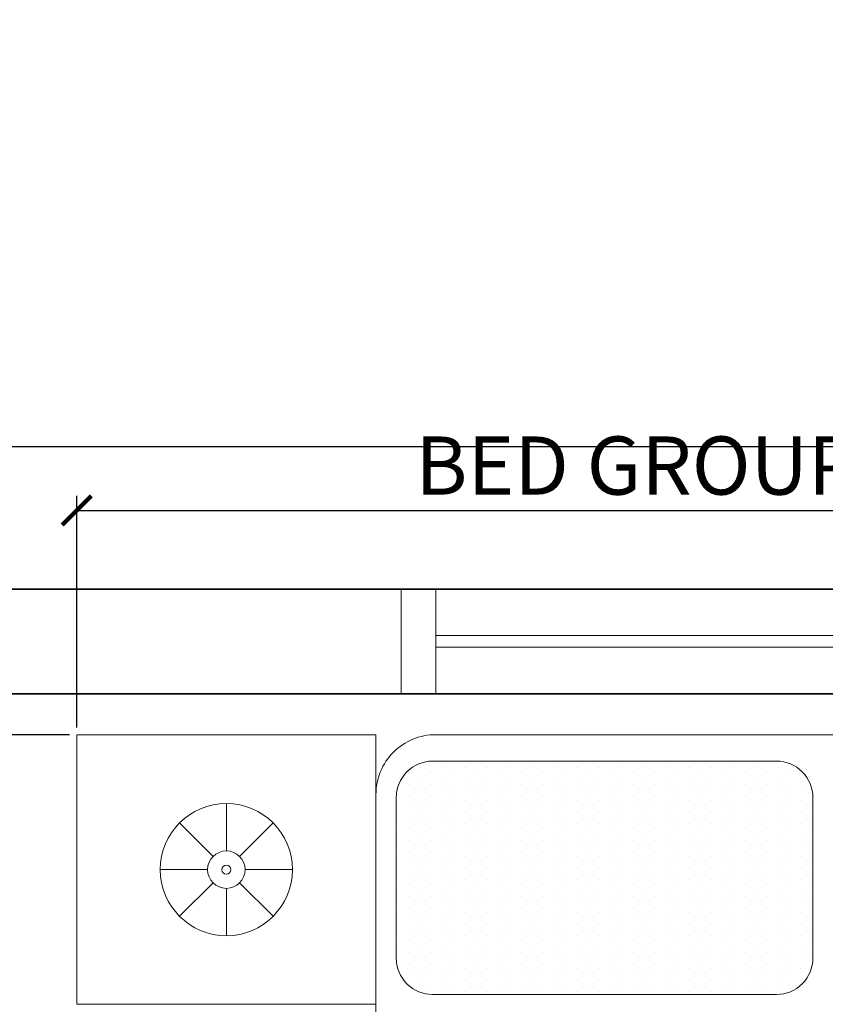
# Model space of a CAD drawing. Units: inches. Extents: x 3283068 to 3284536, y 3240756 to 3241803.
# Tile 10 of 19: x 3283383 to 3283453, y 3241603 to 3241688. Entities that reach past the tile are written whole.
import ezdxf

# ---------------------------------------------------------------- set-up
doc = ezdxf.new("R2010")
doc.units = ezdxf.units.IN
for name, color, linetype, lineweight in [('A-ANNO-DIMS', 2, 'Continuous', 18), ('furniture', 40, 'Continuous', 18), ('wall', 20, 'Continuous', 35), ('window', 100, 'Continuous', 18)]:
    doc.layers.add(name, color=color, linetype=linetype, lineweight=lineweight)
doc.styles.get("Standard").update_dxf_attribs({"font": 'arial.ttf'})
doc.dimstyles.new('ISO-25', dxfattribs={"dimtxt": 5, "dimasz": 2.5, "dimexe": 1.25, "dimexo": 0.625, "dimtad": 1, "dimlunit": 4, "dimtxsty": 'Standard', "dimblk": 'ARCHTICK', "dimcen": 2.5, "dimadec": 0, "dimazin": 0, "dimtfac": 1, "dimtmove": 0, "dimatfit": 3, "dimfxl": 1, "dimarcsym": 0})

# ---------------------------------------------------------------- blocks, each defined once
blk = doc.blocks.new('*X12')
at = {"color": 0}
for p, q in [((266.25, 456.9375), (266.25, 456.9375)), ((266.4375, 457.03125), (266.4375, 457.03125)), ((266.625, 456.9375), (266.625, 456.9375)), ((266.8125, 457.03125), (266.8125, 457.03125)), ((267, 456.9375), (267, 456.9375)), ((267.1875, 457.03125), (267.1875, 457.03125)), ((267.375, 456.9375), (267.375, 456.9375)), ((267.5625, 457.03125), (267.5625, 457.03125)), ((267.75, 456.9375), (267.75, 456.9375)), ((267.9375, 457.03125), (267.9375, 457.03125)), ((268.125, 456.9375), (268.125, 456.9375)), ((268.3125, 457.03125), (268.3125, 457.03125)), ((268.5, 456.9375), (268.5, 456.9375)), ((268.6875, 457.03125), (268.6875, 457.03125)), ((268.875, 456.9375), (268.875, 456.9375)), ((269.0625, 457.03125), (269.0625, 457.03125)), ((269.25, 456.9375), (269.25, 456.9375)), ((269.4375, 457.03125), (269.4375, 457.03125)), ((269.625, 456.9375), (269.625, 456.9375)), ((269.8125, 457.03125), (269.8125, 457.03125)), ((270, 456.9375), (270, 456.9375)), ((270.1875, 457.03125), (270.1875, 457.03125)), ((270.375, 456.9375), (270.375, 456.9375)), ((270.5625, 457.03125), (270.5625, 457.03125)), ((270.75, 456.9375), (270.75, 456.9375)), ((270.9375, 457.03125), (270.9375, 457.03125)), ((271.125, 456.9375), (271.125, 456.9375)), ((271.3125, 457.03125), (271.3125, 457.03125)), ((271.5, 456.9375), (271.5, 456.9375)), ((271.6875, 457.03125), (271.6875, 457.03125)), ((271.875, 456.9375), (271.875, 456.9375)), ((272.0625, 457.03125), (272.0625, 457.03125)), ((272.25, 456.9375), (272.25, 456.9375)), ((266.0625, 456.84375), (266.0625, 456.84375)), ((266.25, 456.75), (266.25, 456.75)), ((266.4375, 456.84375), (266.4375, 456.84375)), ((266.625, 456.75), (266.625, 456.75)), ((266.8125, 456.84375), (266.8125, 456.84375)), ((267, 456.75), (267, 456.75)), ((267.1875, 456.84375), (267.1875, 456.84375)), ((267.375, 456.75), (267.375, 456.75)), ((267.5625, 456.84375), (267.5625, 456.84375)), ((267.75, 456.75), (267.75, 456.75)), ((267.9375, 456.84375), (267.9375, 456.84375)), ((268.125, 456.75), (268.125, 456.75)), ((268.3125, 456.84375), (268.3125, 456.84375)), ((268.5, 456.75), (268.5, 456.75)), ((268.6875, 456.84375), (268.6875, 456.84375)), ((268.875, 456.75), (268.875, 456.75)), ((269.0625, 456.84375), (269.0625, 456.84375)), ((269.25, 456.75), (269.25, 456.75)), ((269.4375, 456.84375), (269.4375, 456.84375)), ((269.625, 456.75), (269.625, 456.75)), ((269.8125, 456.84375), (269.8125, 456.84375)), ((270, 456.75), (270, 456.75)), ((270.1875, 456.84375), (270.1875, 456.84375)), ((270.375, 456.75), (270.375, 456.75)), ((270.5625, 456.84375), (270.5625, 456.84375)), ((270.75, 456.75), (270.75, 456.75)), ((270.9375, 456.84375), (270.9375, 456.84375)), ((271.125, 456.75), (271.125, 456.75)), ((271.3125, 456.84375), (271.3125, 456.84375)), ((271.5, 456.75), (271.5, 456.75)), ((271.6875, 456.84375), (271.6875, 456.84375)), ((271.875, 456.75), (271.875, 456.75)), ((272.0625, 456.84375), (272.0625, 456.84375)), ((272.25, 456.75), (272.25, 456.75)), ((272.4375, 456.84375), (272.4375, 456.84375)), ((272.625, 456.75), (272.625, 456.75)), ((266.0625, 456.65625), (266.0625, 456.65625)), ((266.4375, 456.65625), (266.4375, 456.65625)), ((266.8125, 456.65625), (266.8125, 456.65625)), ((267.1875, 456.65625), (267.1875, 456.65625)), ((267.5625, 456.65625), (267.5625, 456.65625)), ((267.9375, 456.65625), (267.9375, 456.65625)), ((268.3125, 456.65625), (268.3125, 456.65625)), ((268.6875, 456.65625), (268.6875, 456.65625)), ((269.0625, 456.65625), (269.0625, 456.65625)), ((269.4375, 456.65625), (269.4375, 456.65625)), ((269.8125, 456.65625), (269.8125, 456.65625)), ((270.1875, 456.65625), (270.1875, 456.65625)), ((270.5625, 456.65625), (270.5625, 456.65625)), ((270.9375, 456.65625), (270.9375, 456.65625)), ((271.3125, 456.65625), (271.3125, 456.65625)), ((271.6875, 456.65625), (271.6875, 456.65625)), ((272.0625, 456.65625), (272.0625, 456.65625)), ((272.4375, 456.65625), (272.4375, 456.65625)), ((265.875, 456.5625), (265.875, 456.5625)), ((266.0625, 456.46875), (266.0625, 456.46875)), ((266.25, 456.5625), (266.25, 456.5625)), ((266.4375, 456.46875), (266.4375, 456.46875)), ((266.625, 456.5625), (266.625, 456.5625)), ((266.8125, 456.46875), (266.8125, 456.46875)), ((267, 456.5625), (267, 456.5625)), ((267.1875, 456.46875), (267.1875, 456.46875)), ((267.375, 456.5625), (267.375, 456.5625)), ((267.5625, 456.46875), (267.5625, 456.46875)), ((267.75, 456.5625), (267.75, 456.5625)), ((267.9375, 456.46875), (267.9375, 456.46875)), ((268.125, 456.5625), (268.125, 456.5625)), ((268.3125, 456.46875), (268.3125, 456.46875)), ((268.5, 456.5625), (268.5, 456.5625)), ((268.6875, 456.46875), (268.6875, 456.46875)), ((268.875, 456.5625), (268.875, 456.5625)), ((269.0625, 456.46875), (269.0625, 456.46875)), ((269.25, 456.5625), (269.25, 456.5625)), ((269.4375, 456.46875), (269.4375, 456.46875)), ((269.625, 456.5625), (269.625, 456.5625)), ((269.8125, 456.46875), (269.8125, 456.46875)), ((270, 456.5625), (270, 456.5625)), ((270.1875, 456.46875), (270.1875, 456.46875)), ((270.375, 456.5625), (270.375, 456.5625)), ((270.5625, 456.46875), (270.5625, 456.46875)), ((270.75, 456.5625), (270.75, 456.5625)), ((270.9375, 456.46875), (270.9375, 456.46875)), ((271.125, 456.5625), (271.125, 456.5625)), ((271.3125, 456.46875), (271.3125, 456.46875)), ((271.5, 456.5625), (271.5, 456.5625)), ((271.6875, 456.46875), (271.6875, 456.46875)), ((271.875, 456.5625), (271.875, 456.5625)), ((272.0625, 456.46875), (272.0625, 456.46875)), ((272.25, 456.5625), (272.25, 456.5625)), ((272.4375, 456.46875), (272.4375, 456.46875)), ((272.625, 456.5625), (272.625, 456.5625)), ((272.8125, 456.46875), (272.8125, 456.46875)), ((265.875, 456.375), (265.875, 456.375)), ((266.0625, 456.28125), (266.0625, 456.28125)), ((266.25, 456.375), (266.25, 456.375)), ((266.4375, 456.28125), (266.4375, 456.28125)), ((266.625, 456.375), (266.625, 456.375)), ((266.8125, 456.28125), (266.8125, 456.28125)), ((267, 456.375), (267, 456.375)), ((267.1875, 456.28125), (267.1875, 456.28125)), ((267.375, 456.375), (267.375, 456.375)), ((267.5625, 456.28125), (267.5625, 456.28125)), ((267.75, 456.375), (267.75, 456.375)), ((267.9375, 456.28125), (267.9375, 456.28125)), ((268.125, 456.375), (268.125, 456.375)), ((268.3125, 456.28125), (268.3125, 456.28125)), ((268.5, 456.375), (268.5, 456.375)), ((268.6875, 456.28125), (268.6875, 456.28125)), ((268.875, 456.375), (268.875, 456.375)), ((269.0625, 456.28125), (269.0625, 456.28125)), ((269.25, 456.375), (269.25, 456.375)), ((269.4375, 456.28125), (269.4375, 456.28125)), ((269.625, 456.375), (269.625, 456.375)), ((269.8125, 456.28125), (269.8125, 456.28125)), ((270, 456.375), (270, 456.375)), ((270.1875, 456.28125), (270.1875, 456.28125)), ((270.375, 456.375), (270.375, 456.375)), ((270.5625, 456.28125), (270.5625, 456.28125)), ((270.75, 456.375), (270.75, 456.375)), ((270.9375, 456.28125), (270.9375, 456.28125)), ((271.125, 456.375), (271.125, 456.375)), ((271.3125, 456.28125), (271.3125, 456.28125)), ((271.5, 456.375), (271.5, 456.375)), ((271.6875, 456.28125), (271.6875, 456.28125)), ((271.875, 456.375), (271.875, 456.375)), ((272.0625, 456.28125), (272.0625, 456.28125)), ((272.25, 456.375), (272.25, 456.375)), ((272.4375, 456.28125), (272.4375, 456.28125)), ((272.625, 456.375), (272.625, 456.375)), ((272.8125, 456.28125), (272.8125, 456.28125)), ((265.875, 456.1875), (265.875, 456.1875)), ((266.0625, 456.09375), (266.0625, 456.09375)), ((266.25, 456.1875), (266.25, 456.1875)), ((266.4375, 456.09375), (266.4375, 456.09375)), ((266.625, 456.1875), (266.625, 456.1875)), ((266.8125, 456.09375), (266.8125, 456.09375)), ((267, 456.1875), (267, 456.1875)), ((267.1875, 456.09375), (267.1875, 456.09375)), ((267.375, 456.1875), (267.375, 456.1875)), ((267.5625, 456.09375), (267.5625, 456.09375)), ((267.75, 456.1875), (267.75, 456.1875)), ((267.9375, 456.09375), (267.9375, 456.09375)), ((268.125, 456.1875), (268.125, 456.1875)), ((268.3125, 456.09375), (268.3125, 456.09375)), ((268.5, 456.1875), (268.5, 456.1875)), ((268.6875, 456.09375), (268.6875, 456.09375)), ((268.875, 456.1875), (268.875, 456.1875)), ((269.0625, 456.09375), (269.0625, 456.09375)), ((269.25, 456.1875), (269.25, 456.1875)), ((269.4375, 456.09375), (269.4375, 456.09375)), ((269.625, 456.1875), (269.625, 456.1875)), ((269.8125, 456.09375), (269.8125, 456.09375)), ((270, 456.1875), (270, 456.1875)), ((270.1875, 456.09375), (270.1875, 456.09375)), ((270.375, 456.1875), (270.375, 456.1875)), ((270.5625, 456.09375), (270.5625, 456.09375)), ((270.75, 456.1875), (270.75, 456.1875)), ((270.9375, 456.09375), (270.9375, 456.09375)), ((271.125, 456.1875), (271.125, 456.1875)), ((271.3125, 456.09375), (271.3125, 456.09375)), ((271.5, 456.1875), (271.5, 456.1875)), ((271.6875, 456.09375), (271.6875, 456.09375)), ((271.875, 456.1875), (271.875, 456.1875)), ((272.0625, 456.09375), (272.0625, 456.09375)), ((272.25, 456.1875), (272.25, 456.1875)), ((272.4375, 456.09375), (272.4375, 456.09375)), ((272.625, 456.1875), (272.625, 456.1875)), ((272.8125, 456.09375), (272.8125, 456.09375)), ((265.875, 456), (265.875, 456)), ((266.25, 456), (266.25, 456)), ((266.625, 456), (266.625, 456)), ((267, 456), (267, 456)), ((267.375, 456), (267.375, 456)), ((267.75, 456), (267.75, 456)), ((268.125, 456), (268.125, 456)), ((268.5, 456), (268.5, 456)), ((268.875, 456), (268.875, 456)), ((269.25, 456), (269.25, 456)), ((269.625, 456), (269.625, 456)), ((270, 456), (270, 456)), ((270.375, 456), (270.375, 456)), ((270.75, 456), (270.75, 456)), ((271.125, 456), (271.125, 456)), ((271.5, 456), (271.5, 456)), ((271.875, 456), (271.875, 456)), ((272.25, 456), (272.25, 456)), ((272.625, 456), (272.625, 456)), ((265.875, 455.8125), (265.875, 455.8125)), ((266.0625, 455.90625), (266.0625, 455.90625)), ((266.25, 455.8125), (266.25, 455.8125)), ((266.4375, 455.90625), (266.4375, 455.90625)), ((266.625, 455.8125), (266.625, 455.8125)), ((266.8125, 455.90625), (266.8125, 455.90625)), ((267, 455.8125), (267, 455.8125)), ((267.1875, 455.90625), (267.1875, 455.90625)), ((267.375, 455.8125), (267.375, 455.8125)), ((267.5625, 455.90625), (267.5625, 455.90625)), ((267.75, 455.8125), (267.75, 455.8125)), ((267.9375, 455.90625), (267.9375, 455.90625)), ((268.125, 455.8125), (268.125, 455.8125)), ((268.3125, 455.90625), (268.3125, 455.90625)), ((268.5, 455.8125), (268.5, 455.8125)), ((268.6875, 455.90625), (268.6875, 455.90625)), ((268.875, 455.8125), (268.875, 455.8125)), ((269.0625, 455.90625), (269.0625, 455.90625)), ((269.25, 455.8125), (269.25, 455.8125)), ((269.4375, 455.90625), (269.4375, 455.90625)), ((269.625, 455.8125), (269.625, 455.8125)), ((269.8125, 455.90625), (269.8125, 455.90625)), ((270, 455.8125), (270, 455.8125)), ((270.1875, 455.90625), (270.1875, 455.90625)), ((270.375, 455.8125), (270.375, 455.8125)), ((270.5625, 455.90625), (270.5625, 455.90625)), ((270.75, 455.8125), (270.75, 455.8125)), ((270.9375, 455.90625), (270.9375, 455.90625)), ((271.125, 455.8125), (271.125, 455.8125)), ((271.3125, 455.90625), (271.3125, 455.90625)), ((271.5, 455.8125), (271.5, 455.8125)), ((271.6875, 455.90625), (271.6875, 455.90625)), ((271.875, 455.8125), (271.875, 455.8125)), ((272.0625, 455.90625), (272.0625, 455.90625)), ((272.25, 455.8125), (272.25, 455.8125)), ((272.4375, 455.90625), (272.4375, 455.90625)), ((272.625, 455.8125), (272.625, 455.8125)), ((272.8125, 455.90625), (272.8125, 455.90625)), ((265.875, 455.625), (265.875, 455.625)), ((266.0625, 455.71875), (266.0625, 455.71875)), ((266.25, 455.625), (266.25, 455.625)), ((266.4375, 455.71875), (266.4375, 455.71875)), ((266.625, 455.625), (266.625, 455.625)), ((266.8125, 455.71875), (266.8125, 455.71875)), ((267, 455.625), (267, 455.625)), ((267.1875, 455.71875), (267.1875, 455.71875)), ((267.375, 455.625), (267.375, 455.625)), ((267.5625, 455.71875), (267.5625, 455.71875)), ((267.75, 455.625), (267.75, 455.625)), ((267.9375, 455.71875), (267.9375, 455.71875)), ((268.125, 455.625), (268.125, 455.625)), ((268.3125, 455.71875), (268.3125, 455.71875)), ((268.5, 455.625), (268.5, 455.625)), ((268.6875, 455.71875), (268.6875, 455.71875)), ((268.875, 455.625), (268.875, 455.625)), ((269.0625, 455.71875), (269.0625, 455.71875)), ((269.25, 455.625), (269.25, 455.625)), ((269.4375, 455.71875), (269.4375, 455.71875)), ((269.625, 455.625), (269.625, 455.625)), ((269.8125, 455.71875), (269.8125, 455.71875)), ((270, 455.625), (270, 455.625)), ((270.1875, 455.71875), (270.1875, 455.71875)), ((270.375, 455.625), (270.375, 455.625)), ((270.5625, 455.71875), (270.5625, 455.71875)), ((270.75, 455.625), (270.75, 455.625)), ((270.9375, 455.71875), (270.9375, 455.71875)), ((271.125, 455.625), (271.125, 455.625)), ((271.3125, 455.71875), (271.3125, 455.71875)), ((271.5, 455.625), (271.5, 455.625)), ((271.6875, 455.71875), (271.6875, 455.71875)), ((271.875, 455.625), (271.875, 455.625)), ((272.0625, 455.71875), (272.0625, 455.71875)), ((272.25, 455.625), (272.25, 455.625)), ((272.4375, 455.71875), (272.4375, 455.71875)), ((272.625, 455.625), (272.625, 455.625)), ((272.8125, 455.71875), (272.8125, 455.71875)), ((265.875, 455.4375), (265.875, 455.4375)), ((266.0625, 455.53125), (266.0625, 455.53125)), ((266.25, 455.4375), (266.25, 455.4375)), ((266.4375, 455.53125), (266.4375, 455.53125)), ((266.625, 455.4375), (266.625, 455.4375)), ((266.8125, 455.53125), (266.8125, 455.53125)), ((267, 455.4375), (267, 455.4375)), ((267.1875, 455.53125), (267.1875, 455.53125)), ((267.375, 455.4375), (267.375, 455.4375)), ((267.5625, 455.53125), (267.5625, 455.53125)), ((267.75, 455.4375), (267.75, 455.4375)), ((267.9375, 455.53125), (267.9375, 455.53125)), ((268.125, 455.4375), (268.125, 455.4375)), ((268.3125, 455.53125), (268.3125, 455.53125)), ((268.5, 455.4375), (268.5, 455.4375)), ((268.6875, 455.53125), (268.6875, 455.53125)), ((268.875, 455.4375), (268.875, 455.4375)), ((269.0625, 455.53125), (269.0625, 455.53125)), ((269.25, 455.4375), (269.25, 455.4375)), ((269.4375, 455.53125), (269.4375, 455.53125)), ((269.625, 455.4375), (269.625, 455.4375)), ((269.8125, 455.53125), (269.8125, 455.53125)), ((270, 455.4375), (270, 455.4375)), ((270.1875, 455.53125), (270.1875, 455.53125)), ((270.375, 455.4375), (270.375, 455.4375)), ((270.5625, 455.53125), (270.5625, 455.53125)), ((270.75, 455.4375), (270.75, 455.4375)), ((270.9375, 455.53125), (270.9375, 455.53125)), ((271.125, 455.4375), (271.125, 455.4375)), ((271.3125, 455.53125), (271.3125, 455.53125)), ((271.5, 455.4375), (271.5, 455.4375)), ((271.6875, 455.53125), (271.6875, 455.53125)), ((271.875, 455.4375), (271.875, 455.4375)), ((272.0625, 455.53125), (272.0625, 455.53125)), ((272.25, 455.4375), (272.25, 455.4375)), ((272.4375, 455.53125), (272.4375, 455.53125)), ((272.625, 455.4375), (272.625, 455.4375)), ((272.8125, 455.53125), (272.8125, 455.53125)), ((266.0625, 455.34375), (266.0625, 455.34375)), ((266.4375, 455.34375), (266.4375, 455.34375)), ((266.8125, 455.34375), (266.8125, 455.34375)), ((267.1875, 455.34375), (267.1875, 455.34375)), ((267.5625, 455.34375), (267.5625, 455.34375)), ((267.9375, 455.34375), (267.9375, 455.34375)), ((268.3125, 455.34375), (268.3125, 455.34375)), ((268.6875, 455.34375), (268.6875, 455.34375)), ((269.0625, 455.34375), (269.0625, 455.34375)), ((269.4375, 455.34375), (269.4375, 455.34375)), ((269.8125, 455.34375), (269.8125, 455.34375)), ((270.1875, 455.34375), (270.1875, 455.34375)), ((270.5625, 455.34375), (270.5625, 455.34375)), ((270.9375, 455.34375), (270.9375, 455.34375)), ((271.3125, 455.34375), (271.3125, 455.34375)), ((271.6875, 455.34375), (271.6875, 455.34375)), ((272.0625, 455.34375), (272.0625, 455.34375)), ((272.4375, 455.34375), (272.4375, 455.34375)), ((272.8125, 455.34375), (272.8125, 455.34375)), ((265.875, 455.25), (265.875, 455.25)), ((266.0625, 455.15625), (266.0625, 455.15625)), ((266.25, 455.25), (266.25, 455.25)), ((266.4375, 455.15625), (266.4375, 455.15625)), ((266.625, 455.25), (266.625, 455.25)), ((266.8125, 455.15625), (266.8125, 455.15625)), ((267, 455.25), (267, 455.25)), ((267.1875, 455.15625), (267.1875, 455.15625)), ((267.375, 455.25), (267.375, 455.25)), ((267.5625, 455.15625), (267.5625, 455.15625)), ((267.75, 455.25), (267.75, 455.25)), ((267.9375, 455.15625), (267.9375, 455.15625)), ((268.125, 455.25), (268.125, 455.25)), ((268.3125, 455.15625), (268.3125, 455.15625)), ((268.5, 455.25), (268.5, 455.25)), ((268.6875, 455.15625), (268.6875, 455.15625)), ((268.875, 455.25), (268.875, 455.25)), ((269.0625, 455.15625), (269.0625, 455.15625)), ((269.25, 455.25), (269.25, 455.25)), ((269.4375, 455.15625), (269.4375, 455.15625)), ((269.625, 455.25), (269.625, 455.25)), ((269.8125, 455.15625), (269.8125, 455.15625)), ((270, 455.25), (270, 455.25)), ((270.1875, 455.15625), (270.1875, 455.15625)), ((270.375, 455.25), (270.375, 455.25)), ((270.5625, 455.15625), (270.5625, 455.15625)), ((270.75, 455.25), (270.75, 455.25)), ((270.9375, 455.15625), (270.9375, 455.15625)), ((271.125, 455.25), (271.125, 455.25)), ((271.3125, 455.15625), (271.3125, 455.15625)), ((271.5, 455.25), (271.5, 455.25)), ((271.6875, 455.15625), (271.6875, 455.15625)), ((271.875, 455.25), (271.875, 455.25)), ((272.0625, 455.15625), (272.0625, 455.15625)), ((272.25, 455.25), (272.25, 455.25)), ((272.4375, 455.15625), (272.4375, 455.15625)), ((272.625, 455.25), (272.625, 455.25)), ((272.8125, 455.15625), (272.8125, 455.15625)), ((265.875, 455.0625), (265.875, 455.0625)), ((266.0625, 454.96875), (266.0625, 454.96875)), ((266.25, 455.0625), (266.25, 455.0625)), ((266.4375, 454.96875), (266.4375, 454.96875)), ((266.625, 455.0625), (266.625, 455.0625)), ((266.8125, 454.96875), (266.8125, 454.96875)), ((267, 455.0625), (267, 455.0625)), ((267.1875, 454.96875), (267.1875, 454.96875)), ((267.375, 455.0625), (267.375, 455.0625)), ((267.5625, 454.96875), (267.5625, 454.96875)), ((267.75, 455.0625), (267.75, 455.0625)), ((267.9375, 454.96875), (267.9375, 454.96875)), ((268.125, 455.0625), (268.125, 455.0625)), ((268.3125, 454.96875), (268.3125, 454.96875)), ((268.5, 455.0625), (268.5, 455.0625)), ((268.6875, 454.96875), (268.6875, 454.96875)), ((268.875, 455.0625), (268.875, 455.0625)), ((269.0625, 454.96875), (269.0625, 454.96875)), ((269.25, 455.0625), (269.25, 455.0625)), ((269.4375, 454.96875), (269.4375, 454.96875)), ((269.625, 455.0625), (269.625, 455.0625)), ((269.8125, 454.96875), (269.8125, 454.96875)), ((270, 455.0625), (270, 455.0625)), ((270.1875, 454.96875), (270.1875, 454.96875)), ((270.375, 455.0625), (270.375, 455.0625)), ((270.5625, 454.96875), (270.5625, 454.96875)), ((270.75, 455.0625), (270.75, 455.0625)), ((270.9375, 454.96875), (270.9375, 454.96875)), ((271.125, 455.0625), (271.125, 455.0625)), ((271.3125, 454.96875), (271.3125, 454.96875)), ((271.5, 455.0625), (271.5, 455.0625)), ((271.6875, 454.96875), (271.6875, 454.96875)), ((271.875, 455.0625), (271.875, 455.0625)), ((272.0625, 454.96875), (272.0625, 454.96875)), ((272.25, 455.0625), (272.25, 455.0625)), ((272.4375, 454.96875), (272.4375, 454.96875)), ((272.625, 455.0625), (272.625, 455.0625)), ((272.8125, 454.96875), (272.8125, 454.96875)), ((265.875, 454.875), (265.875, 454.875)), ((266.0625, 454.78125), (266.0625, 454.78125)), ((266.25, 454.875), (266.25, 454.875)), ((266.4375, 454.78125), (266.4375, 454.78125)), ((266.625, 454.875), (266.625, 454.875)), ((266.8125, 454.78125), (266.8125, 454.78125)), ((267, 454.875), (267, 454.875)), ((267.1875, 454.78125), (267.1875, 454.78125)), ((267.375, 454.875), (267.375, 454.875)), ((267.5625, 454.78125), (267.5625, 454.78125)), ((267.75, 454.875), (267.75, 454.875)), ((267.9375, 454.78125), (267.9375, 454.78125)), ((268.125, 454.875), (268.125, 454.875)), ((268.3125, 454.78125), (268.3125, 454.78125)), ((268.5, 454.875), (268.5, 454.875)), ((268.6875, 454.78125), (268.6875, 454.78125)), ((268.875, 454.875), (268.875, 454.875)), ((269.0625, 454.78125), (269.0625, 454.78125)), ((269.25, 454.875), (269.25, 454.875)), ((269.4375, 454.78125), (269.4375, 454.78125)), ((269.625, 454.875), (269.625, 454.875)), ((269.8125, 454.78125), (269.8125, 454.78125)), ((270, 454.875), (270, 454.875)), ((270.1875, 454.78125), (270.1875, 454.78125)), ((270.375, 454.875), (270.375, 454.875)), ((270.5625, 454.78125), (270.5625, 454.78125)), ((270.75, 454.875), (270.75, 454.875)), ((270.9375, 454.78125), (270.9375, 454.78125)), ((271.125, 454.875), (271.125, 454.875)), ((271.3125, 454.78125), (271.3125, 454.78125)), ((271.5, 454.875), (271.5, 454.875)), ((271.6875, 454.78125), (271.6875, 454.78125)), ((271.875, 454.875), (271.875, 454.875)), ((272.0625, 454.78125), (272.0625, 454.78125)), ((272.25, 454.875), (272.25, 454.875)), ((272.4375, 454.78125), (272.4375, 454.78125)), ((272.625, 454.875), (272.625, 454.875)), ((272.8125, 454.78125), (272.8125, 454.78125)), ((265.875, 454.6875), (265.875, 454.6875)), ((266.25, 454.6875), (266.25, 454.6875)), ((266.625, 454.6875), (266.625, 454.6875)), ((267, 454.6875), (267, 454.6875)), ((267.375, 454.6875), (267.375, 454.6875)), ((267.75, 454.6875), (267.75, 454.6875)), ((268.125, 454.6875), (268.125, 454.6875)), ((268.5, 454.6875), (268.5, 454.6875)), ((268.875, 454.6875), (268.875, 454.6875)), ((269.25, 454.6875), (269.25, 454.6875)), ((269.625, 454.6875), (269.625, 454.6875)), ((270, 454.6875), (270, 454.6875)), ((270.375, 454.6875), (270.375, 454.6875)), ((270.75, 454.6875), (270.75, 454.6875)), ((271.125, 454.6875), (271.125, 454.6875)), ((271.5, 454.6875), (271.5, 454.6875)), ((271.875, 454.6875), (271.875, 454.6875)), ((272.25, 454.6875), (272.25, 454.6875)), ((272.625, 454.6875), (272.625, 454.6875)), ((265.875, 454.5), (265.875, 454.5)), ((266.0625, 454.59375), (266.0625, 454.59375)), ((266.25, 454.5), (266.25, 454.5)), ((266.4375, 454.59375), (266.4375, 454.59375)), ((266.625, 454.5), (266.625, 454.5)), ((266.8125, 454.59375), (266.8125, 454.59375)), ((267, 454.5), (267, 454.5)), ((267.1875, 454.59375), (267.1875, 454.59375)), ((267.375, 454.5), (267.375, 454.5)), ((267.5625, 454.59375), (267.5625, 454.59375)), ((267.75, 454.5), (267.75, 454.5)), ((267.9375, 454.59375), (267.9375, 454.59375)), ((268.125, 454.5), (268.125, 454.5)), ((268.3125, 454.59375), (268.3125, 454.59375)), ((268.5, 454.5), (268.5, 454.5)), ((268.6875, 454.59375), (268.6875, 454.59375)), ((268.875, 454.5), (268.875, 454.5)), ((269.0625, 454.59375), (269.0625, 454.59375)), ((269.25, 454.5), (269.25, 454.5)), ((269.4375, 454.59375), (269.4375, 454.59375)), ((269.625, 454.5), (269.625, 454.5)), ((269.8125, 454.59375), (269.8125, 454.59375)), ((270, 454.5), (270, 454.5)), ((270.1875, 454.59375), (270.1875, 454.59375)), ((270.375, 454.5), (270.375, 454.5)), ((270.5625, 454.59375), (270.5625, 454.59375)), ((270.75, 454.5), (270.75, 454.5)), ((270.9375, 454.59375), (270.9375, 454.59375)), ((271.125, 454.5), (271.125, 454.5)), ((271.3125, 454.59375), (271.3125, 454.59375)), ((271.5, 454.5), (271.5, 454.5)), ((271.6875, 454.59375), (271.6875, 454.59375)), ((271.875, 454.5), (271.875, 454.5)), ((272.0625, 454.59375), (272.0625, 454.59375)), ((272.25, 454.5), (272.25, 454.5)), ((272.4375, 454.59375), (272.4375, 454.59375)), ((272.625, 454.5), (272.625, 454.5)), ((272.8125, 454.59375), (272.8125, 454.59375)), ((265.875, 454.3125), (265.875, 454.3125)), ((266.0625, 454.40625), (266.0625, 454.40625)), ((266.25, 454.3125), (266.25, 454.3125)), ((266.4375, 454.40625), (266.4375, 454.40625)), ((266.625, 454.3125), (266.625, 454.3125)), ((266.8125, 454.40625), (266.8125, 454.40625)), ((267, 454.3125), (267, 454.3125)), ((267.1875, 454.40625), (267.1875, 454.40625)), ((267.375, 454.3125), (267.375, 454.3125)), ((267.5625, 454.40625), (267.5625, 454.40625)), ((267.75, 454.3125), (267.75, 454.3125)), ((267.9375, 454.40625), (267.9375, 454.40625)), ((268.125, 454.3125), (268.125, 454.3125)), ((268.3125, 454.40625), (268.3125, 454.40625)), ((268.5, 454.3125), (268.5, 454.3125)), ((268.6875, 454.40625), (268.6875, 454.40625)), ((268.875, 454.3125), (268.875, 454.3125)), ((269.0625, 454.40625), (269.0625, 454.40625)), ((269.25, 454.3125), (269.25, 454.3125)), ((269.4375, 454.40625), (269.4375, 454.40625)), ((269.625, 454.3125), (269.625, 454.3125)), ((269.8125, 454.40625), (269.8125, 454.40625)), ((270, 454.3125), (270, 454.3125)), ((270.1875, 454.40625), (270.1875, 454.40625)), ((270.375, 454.3125), (270.375, 454.3125)), ((270.5625, 454.40625), (270.5625, 454.40625)), ((270.75, 454.3125), (270.75, 454.3125)), ((270.9375, 454.40625), (270.9375, 454.40625)), ((271.125, 454.3125), (271.125, 454.3125)), ((271.3125, 454.40625), (271.3125, 454.40625)), ((271.5, 454.3125), (271.5, 454.3125)), ((271.6875, 454.40625), (271.6875, 454.40625)), ((271.875, 454.3125), (271.875, 454.3125)), ((272.0625, 454.40625), (272.0625, 454.40625)), ((272.25, 454.3125), (272.25, 454.3125)), ((272.4375, 454.40625), (272.4375, 454.40625)), ((272.625, 454.3125), (272.625, 454.3125)), ((272.8125, 454.40625), (272.8125, 454.40625)), ((265.875, 454.125), (265.875, 454.125)), ((266.0625, 454.21875), (266.0625, 454.21875)), ((266.25, 454.125), (266.25, 454.125)), ((266.4375, 454.21875), (266.4375, 454.21875)), ((266.625, 454.125), (266.625, 454.125)), ((266.8125, 454.21875), (266.8125, 454.21875)), ((267, 454.125), (267, 454.125)), ((267.1875, 454.21875), (267.1875, 454.21875)), ((267.375, 454.125), (267.375, 454.125)), ((267.5625, 454.21875), (267.5625, 454.21875)), ((267.75, 454.125), (267.75, 454.125)), ((267.9375, 454.21875), (267.9375, 454.21875)), ((268.125, 454.125), (268.125, 454.125)), ((268.3125, 454.21875), (268.3125, 454.21875)), ((268.5, 454.125), (268.5, 454.125)), ((268.6875, 454.21875), (268.6875, 454.21875)), ((268.875, 454.125), (268.875, 454.125)), ((269.0625, 454.21875), (269.0625, 454.21875)), ((269.25, 454.125), (269.25, 454.125)), ((269.4375, 454.21875), (269.4375, 454.21875)), ((269.625, 454.125), (269.625, 454.125)), ((269.8125, 454.21875), (269.8125, 454.21875)), ((270, 454.125), (270, 454.125)), ((270.1875, 454.21875), (270.1875, 454.21875)), ((270.375, 454.125), (270.375, 454.125)), ((270.5625, 454.21875), (270.5625, 454.21875)), ((270.75, 454.125), (270.75, 454.125)), ((270.9375, 454.21875), (270.9375, 454.21875)), ((271.125, 454.125), (271.125, 454.125)), ((271.3125, 454.21875), (271.3125, 454.21875)), ((271.5, 454.125), (271.5, 454.125)), ((271.6875, 454.21875), (271.6875, 454.21875)), ((271.875, 454.125), (271.875, 454.125)), ((272.0625, 454.21875), (272.0625, 454.21875)), ((272.25, 454.125), (272.25, 454.125)), ((272.4375, 454.21875), (272.4375, 454.21875)), ((272.625, 454.125), (272.625, 454.125)), ((272.8125, 454.21875), (272.8125, 454.21875)), ((266.0625, 454.03125), (266.0625, 454.03125)), ((266.4375, 454.03125), (266.4375, 454.03125)), ((266.8125, 454.03125), (266.8125, 454.03125)), ((267.1875, 454.03125), (267.1875, 454.03125)), ((267.5625, 454.03125), (267.5625, 454.03125)), ((267.9375, 454.03125), (267.9375, 454.03125)), ((268.3125, 454.03125), (268.3125, 454.03125)), ((268.6875, 454.03125), (268.6875, 454.03125)), ((269.0625, 454.03125), (269.0625, 454.03125)), ((269.4375, 454.03125), (269.4375, 454.03125)), ((269.8125, 454.03125), (269.8125, 454.03125)), ((270.1875, 454.03125), (270.1875, 454.03125)), ((270.5625, 454.03125), (270.5625, 454.03125)), ((270.9375, 454.03125), (270.9375, 454.03125)), ((271.3125, 454.03125), (271.3125, 454.03125)), ((271.6875, 454.03125), (271.6875, 454.03125)), ((272.0625, 454.03125), (272.0625, 454.03125)), ((272.4375, 454.03125), (272.4375, 454.03125)), ((272.8125, 454.03125), (272.8125, 454.03125)), ((265.875, 453.9375), (265.875, 453.9375)), ((266.0625, 453.84375), (266.0625, 453.84375)), ((266.25, 453.9375), (266.25, 453.9375)), ((266.4375, 453.84375), (266.4375, 453.84375)), ((266.625, 453.9375), (266.625, 453.9375)), ((266.8125, 453.84375), (266.8125, 453.84375)), ((267, 453.9375), (267, 453.9375)), ((267.1875, 453.84375), (267.1875, 453.84375)), ((267.375, 453.9375), (267.375, 453.9375)), ((267.5625, 453.84375), (267.5625, 453.84375)), ((267.75, 453.9375), (267.75, 453.9375)), ((267.9375, 453.84375), (267.9375, 453.84375)), ((268.125, 453.9375), (268.125, 453.9375)), ((268.3125, 453.84375), (268.3125, 453.84375)), ((268.5, 453.9375), (268.5, 453.9375)), ((268.6875, 453.84375), (268.6875, 453.84375)), ((268.875, 453.9375), (268.875, 453.9375)), ((269.0625, 453.84375), (269.0625, 453.84375)), ((269.25, 453.9375), (269.25, 453.9375)), ((269.4375, 453.84375), (269.4375, 453.84375)), ((269.625, 453.9375), (269.625, 453.9375)), ((269.8125, 453.84375), (269.8125, 453.84375)), ((270, 453.9375), (270, 453.9375)), ((270.1875, 453.84375), (270.1875, 453.84375)), ((270.375, 453.9375), (270.375, 453.9375)), ((270.5625, 453.84375), (270.5625, 453.84375)), ((270.75, 453.9375), (270.75, 453.9375)), ((270.9375, 453.84375), (270.9375, 453.84375)), ((271.125, 453.9375), (271.125, 453.9375)), ((271.3125, 453.84375), (271.3125, 453.84375)), ((271.5, 453.9375), (271.5, 453.9375)), ((271.6875, 453.84375), (271.6875, 453.84375)), ((271.875, 453.9375), (271.875, 453.9375)), ((272.0625, 453.84375), (272.0625, 453.84375)), ((272.25, 453.9375), (272.25, 453.9375)), ((272.4375, 453.84375), (272.4375, 453.84375)), ((272.625, 453.9375), (272.625, 453.9375)), ((272.8125, 453.84375), (272.8125, 453.84375)), ((265.875, 453.75), (265.875, 453.75)), ((266.0625, 453.65625), (266.0625, 453.65625)), ((266.25, 453.75), (266.25, 453.75)), ((266.4375, 453.65625), (266.4375, 453.65625)), ((266.625, 453.75), (266.625, 453.75)), ((266.8125, 453.65625), (266.8125, 453.65625)), ((267, 453.75), (267, 453.75)), ((267.1875, 453.65625), (267.1875, 453.65625)), ((267.375, 453.75), (267.375, 453.75)), ((267.5625, 453.65625), (267.5625, 453.65625)), ((267.75, 453.75), (267.75, 453.75)), ((267.9375, 453.65625), (267.9375, 453.65625)), ((268.125, 453.75), (268.125, 453.75)), ((268.3125, 453.65625), (268.3125, 453.65625)), ((268.5, 453.75), (268.5, 453.75)), ((268.6875, 453.65625), (268.6875, 453.65625)), ((268.875, 453.75), (268.875, 453.75)), ((269.0625, 453.65625), (269.0625, 453.65625)), ((269.25, 453.75), (269.25, 453.75)), ((269.4375, 453.65625), (269.4375, 453.65625)), ((269.625, 453.75), (269.625, 453.75)), ((269.8125, 453.65625), (269.8125, 453.65625)), ((270, 453.75), (270, 453.75)), ((270.1875, 453.65625), (270.1875, 453.65625)), ((270.375, 453.75), (270.375, 453.75)), ((270.5625, 453.65625), (270.5625, 453.65625)), ((270.75, 453.75), (270.75, 453.75)), ((270.9375, 453.65625), (270.9375, 453.65625)), ((271.125, 453.75), (271.125, 453.75)), ((271.3125, 453.65625), (271.3125, 453.65625)), ((271.5, 453.75), (271.5, 453.75)), ((271.6875, 453.65625), (271.6875, 453.65625)), ((271.875, 453.75), (271.875, 453.75)), ((272.0625, 453.65625), (272.0625, 453.65625)), ((272.25, 453.75), (272.25, 453.75)), ((272.4375, 453.65625), (272.4375, 453.65625)), ((272.625, 453.75), (272.625, 453.75)), ((272.8125, 453.65625), (272.8125, 453.65625)), ((266.0625, 453.46875), (266.0625, 453.46875)), ((266.25, 453.5625), (266.25, 453.5625)), ((266.4375, 453.46875), (266.4375, 453.46875)), ((266.625, 453.5625), (266.625, 453.5625)), ((266.8125, 453.46875), (266.8125, 453.46875)), ((267, 453.5625), (267, 453.5625)), ((267.1875, 453.46875), (267.1875, 453.46875)), ((267.375, 453.5625), (267.375, 453.5625)), ((267.5625, 453.46875), (267.5625, 453.46875)), ((267.75, 453.5625), (267.75, 453.5625)), ((267.9375, 453.46875), (267.9375, 453.46875)), ((268.125, 453.5625), (268.125, 453.5625)), ((268.3125, 453.46875), (268.3125, 453.46875)), ((268.5, 453.5625), (268.5, 453.5625)), ((268.6875, 453.46875), (268.6875, 453.46875)), ((268.875, 453.5625), (268.875, 453.5625)), ((269.0625, 453.46875), (269.0625, 453.46875)), ((269.25, 453.5625), (269.25, 453.5625)), ((269.4375, 453.46875), (269.4375, 453.46875)), ((269.625, 453.5625), (269.625, 453.5625)), ((269.8125, 453.46875), (269.8125, 453.46875)), ((270, 453.5625), (270, 453.5625)), ((270.1875, 453.46875), (270.1875, 453.46875)), ((270.375, 453.5625), (270.375, 453.5625)), ((270.5625, 453.46875), (270.5625, 453.46875)), ((270.75, 453.5625), (270.75, 453.5625)), ((270.9375, 453.46875), (270.9375, 453.46875)), ((271.125, 453.5625), (271.125, 453.5625)), ((271.3125, 453.46875), (271.3125, 453.46875)), ((271.5, 453.5625), (271.5, 453.5625)), ((271.6875, 453.46875), (271.6875, 453.46875)), ((271.875, 453.5625), (271.875, 453.5625)), ((272.0625, 453.46875), (272.0625, 453.46875)), ((272.25, 453.5625), (272.25, 453.5625)), ((272.4375, 453.46875), (272.4375, 453.46875)), ((272.625, 453.5625), (272.625, 453.5625)), ((266.25, 453.375), (266.25, 453.375)), ((266.625, 453.375), (266.625, 453.375)), ((267, 453.375), (267, 453.375)), ((267.375, 453.375), (267.375, 453.375)), ((267.75, 453.375), (267.75, 453.375)), ((268.125, 453.375), (268.125, 453.375)), ((268.5, 453.375), (268.5, 453.375)), ((268.875, 453.375), (268.875, 453.375)), ((269.25, 453.375), (269.25, 453.375)), ((269.625, 453.375), (269.625, 453.375)), ((270, 453.375), (270, 453.375)), ((270.375, 453.375), (270.375, 453.375)), ((270.75, 453.375), (270.75, 453.375)), ((271.125, 453.375), (271.125, 453.375)), ((271.5, 453.375), (271.5, 453.375)), ((271.875, 453.375), (271.875, 453.375)), ((272.25, 453.375), (272.25, 453.375)), ((272.625, 453.375), (272.625, 453.375)), ((266.0625, 453.28125), (266.0625, 453.28125)), ((266.25, 453.1875), (266.25, 453.1875)), ((266.4375, 453.28125), (266.4375, 453.28125)), ((266.625, 453.1875), (266.625, 453.1875)), ((266.8125, 453.28125), (266.8125, 453.28125)), ((267, 453.1875), (267, 453.1875)), ((267.1875, 453.28125), (267.1875, 453.28125)), ((267.375, 453.1875), (267.375, 453.1875)), ((267.5625, 453.28125), (267.5625, 453.28125)), ((267.75, 453.1875), (267.75, 453.1875)), ((267.9375, 453.28125), (267.9375, 453.28125)), ((268.125, 453.1875), (268.125, 453.1875)), ((268.3125, 453.28125), (268.3125, 453.28125)), ((268.5, 453.1875), (268.5, 453.1875)), ((268.6875, 453.28125), (268.6875, 453.28125)), ((268.875, 453.1875), (268.875, 453.1875)), ((269.0625, 453.28125), (269.0625, 453.28125)), ((269.25, 453.1875), (269.25, 453.1875)), ((269.4375, 453.28125), (269.4375, 453.28125)), ((269.625, 453.1875), (269.625, 453.1875)), ((269.8125, 453.28125), (269.8125, 453.28125)), ((270, 453.1875), (270, 453.1875)), ((270.1875, 453.28125), (270.1875, 453.28125)), ((270.375, 453.1875), (270.375, 453.1875)), ((270.5625, 453.28125), (270.5625, 453.28125)), ((270.75, 453.1875), (270.75, 453.1875)), ((270.9375, 453.28125), (270.9375, 453.28125)), ((271.125, 453.1875), (271.125, 453.1875)), ((271.3125, 453.28125), (271.3125, 453.28125)), ((271.5, 453.1875), (271.5, 453.1875)), ((271.6875, 453.28125), (271.6875, 453.28125)), ((271.875, 453.1875), (271.875, 453.1875)), ((272.0625, 453.28125), (272.0625, 453.28125)), ((272.25, 453.1875), (272.25, 453.1875)), ((272.4375, 453.28125), (272.4375, 453.28125))]:
    blk.add_line(p, q, dxfattribs=at)
blk = doc.blocks.new('A$C52E67D0D')
at = {"layer": 'furniture'}
for p, q in [((250.5, 1605.5), (250.5, 1684.7)), ((228.3, 1596.3), (172.3, 1652.3)), ((272.7, 1596.3), (328.7, 1652.3)), ((219.1, 1574.1), (139.9, 1574.1)), ((281.9, 1574.1), (361.1, 1574.1)), ((228.3, 1551.9), (172.3, 1495.9)), ((272.7, 1551.9), (328.7, 1495.9)), ((250.5, 1542.8), (250.5, 1463.5))]:
    blk.add_line(p, q, dxfattribs=at)
blk.add_lwpolyline([(501, 1348.6), (501, 1799.6), (0, 1799.6), (0, 1348.6)], close=True, dxfattribs=at)
for points in [[(1901, 0), (601, 0, -0.414214), (501, 100), (501, 1700, -0.414214), (601, 1800), (1901, 1800, -0.414214), (2001, 1700), (2001, 100, -0.414214)], [(1171.8, 1365.1), (595.8, 1365.1, -0.414214), (535, 1425.9), (535, 1694.8, -0.414214), (595.8, 1755.7), (1171.8, 1755.7, -0.414214), (1232.6, 1694.8), (1232.6, 1425.9, -0.414214)]]:
    blk.add_lwpolyline(points, format="xyb", close=True, dxfattribs=at)
for radius in [110.6, 31.4, 7.46]:
    blk.add_circle((250.5, 1574.1), radius, dxfattribs=at)
for centre, radius, start, end in [((1888.6, -1664.5), 3015.3, 87.8642, 117.4001), ((3101, -1685.8), 3227.7, 109.926, 135.3977)]:
    blk.add_arc(centre, radius, start, end, dxfattribs=at)
at = {"layer": 'furniture', "xscale": 100, "yscale": 100, "zscale": 100}
blk.add_blockref('*X12', (-26050, -43948.2), dxfattribs=at)
blk = doc.blocks.new('_ArchTick')
at = {"color": 0, "linetype": 'ByBlock', "const_width": 0.15}
blk.add_lwpolyline([(-0.5, -0.5), (0.5, 0.5)], dxfattribs=at)
blk = doc.blocks.new('*D25')
at = {"layer": 'A-ANNO-DIMS', "color": 0, "lineweight": -2, "transparency": 16777216}
for p, q in [((3283339.589, 3241639.727), (3283339.589, 3241652.584)), ((3284236.589, 3241639.727), (3284236.589, 3241652.584)), ((3283339.589, 3241651.334), (3284236.589, 3241651.334))]:
    blk.add_line(p, q, dxfattribs=at)
at = {"layer": 'Defpoints', "color": 0, "transparency": 16777216}
for p in [(3284236.589, 3241651.334), (3283339.589, 3241639.102), (3284236.589, 3241639.102)]:
    blk.add_point(p, dxfattribs=at)
at = {"layer": 'A-ANNO-DIMS', "color": 0, "lineweight": -2, "transparency": 16777216, "xscale": 2.5, "yscale": 2.5, "zscale": 2.5, "rotation": 180}
blk.add_blockref('_ArchTick', (3283339.589, 3241651.334), dxfattribs=at)
at = {"layer": 'A-ANNO-DIMS', "color": 0, "lineweight": -2, "transparency": 16777216, "xscale": 2.5, "yscale": 2.5, "zscale": 2.5}
blk.add_blockref('_ArchTick', (3284236.589, 3241651.334), dxfattribs=at)
at = {"layer": 'A-ANNO-DIMS', "color": 0, "transparency": 16777216, "insert": (3283788.089, 3241654.512), "char_height": 5, "attachment_point": 5}
blk.add_mtext('74\'-9"', dxfattribs=at)
blk = doc.blocks.new('WIN-48IN-9IN-WALL')
for p, q in [((0, 9), (48, 9)), ((0, 0), (0, 9)), ((3, 0), (3, 9)), ((45, 9), (45, 0)), ((48, 9), (48, 0)), ((3, 5), (45, 5)), ((3, 4), (45, 4)), ((48, 0), (0, 0))]:
    blk.add_line(p, q)
blk = doc.blocks.new('*D57')
at = {"layer": 'A-ANNO-DIMS', "color": 0, "lineweight": -2, "transparency": 16777216}
for p, q in [((3283388.229, 3241627.215), (3283388.229, 3241647.098)), ((3283516.614, 3241627.215), (3283516.614, 3241647.098)), ((3283388.229, 3241645.848), (3283516.614, 3241645.848))]:
    blk.add_line(p, q, dxfattribs=at)
at = {"layer": 'Defpoints', "color": 0, "transparency": 16777216}
for p in [(3283516.614, 3241645.848), (3283388.229, 3241626.59), (3283516.614, 3241626.59)]:
    blk.add_point(p, dxfattribs=at)
at = {"layer": 'A-ANNO-DIMS', "color": 0, "lineweight": -2, "transparency": 16777216, "xscale": 2.5, "yscale": 2.5, "zscale": 2.5, "rotation": 180}
blk.add_blockref('_ArchTick', (3283388.229, 3241645.848), dxfattribs=at)
at = {"layer": 'A-ANNO-DIMS', "color": 0, "lineweight": -2, "transparency": 16777216, "xscale": 2.5, "yscale": 2.5, "zscale": 2.5}
blk.add_blockref('_ArchTick', (3283516.614, 3241645.848), dxfattribs=at)
at = {"layer": 'A-ANNO-DIMS', "color": 0, "transparency": 16777216, "insert": (3283452.421, 3241649.06), "char_height": 5, "attachment_point": 5}
blk.add_mtext('BED GROUP 10\'-8 1/2"', dxfattribs=at)
blk = doc.blocks.new('*D58')
at = {"layer": 'A-ANNO-DIMS', "color": 0, "lineweight": -2, "transparency": 16777216}
for p, q in [((3283387.604, 3241626.59), (3283367.721, 3241626.59)), ((3283368.971, 3241534.227), (3283368.971, 3241626.59)), ((3283387.604, 3241534.227), (3283367.721, 3241534.227))]:
    blk.add_line(p, q, dxfattribs=at)
at = {"layer": 'Defpoints', "color": 0, "transparency": 16777216}
for p in [(3283368.971, 3241626.59), (3283388.229, 3241626.59), (3283388.229, 3241534.227)]:
    blk.add_point(p, dxfattribs=at)
at = {"layer": 'A-ANNO-DIMS', "color": 0, "lineweight": -2, "transparency": 16777216, "xscale": 2.5, "yscale": 2.5, "zscale": 2.5}
for p, rotation in [((3283368.971, 3241626.59), 90), ((3283368.971, 3241534.227), 270)]:
    blk.add_blockref('_ArchTick', p, dxfattribs=dict(at, rotation=rotation))
at = {"layer": 'A-ANNO-DIMS', "color": 0, "transparency": 16777216, "insert": (3283365.761, 3241580.409), "char_height": 5, "attachment_point": 5, "rotation": 90}
blk.add_mtext('7\'-8 1/2"', dxfattribs=at)
blk = doc.blocks.new('*D63')
at = {"layer": 'A-ANNO-DIMS', "color": 0, "lineweight": -2, "transparency": 16777216}
for p, q in [((3283248.089, 3241083.227), (3283248.089, 3241798.077)), ((3284328.089, 3241083.227), (3284328.089, 3241798.077)), ((3283248.089, 3241796.827), (3284328.089, 3241796.827))]:
    blk.add_line(p, q, dxfattribs=at)
at = {"layer": 'Defpoints', "color": 0, "transparency": 16777216}
for p in [(3284328.089, 3241796.827), (3283248.089, 3241082.602), (3284328.089, 3241082.602)]:
    blk.add_point(p, dxfattribs=at)
at = {"layer": 'A-ANNO-DIMS', "color": 0, "lineweight": -2, "transparency": 16777216, "xscale": 2.5, "yscale": 2.5, "zscale": 2.5, "rotation": 180}
blk.add_blockref('_ArchTick', (3283248.089, 3241796.827), dxfattribs=at)
at = {"layer": 'A-ANNO-DIMS', "color": 0, "lineweight": -2, "transparency": 16777216, "xscale": 2.5, "yscale": 2.5, "zscale": 2.5}
blk.add_blockref('_ArchTick', (3284328.089, 3241796.827), dxfattribs=at)
at = {"layer": 'A-ANNO-DIMS', "color": 0, "transparency": 16777216, "insert": (3283788.089, 3241800.005), "char_height": 5, "attachment_point": 5}
blk.add_mtext('90\'-0"', dxfattribs=at)

msp = doc.modelspace()

# ---------------------------------------------------------------- linework, layer by layer
at = {"layer": 'wall'}
for p, q in [((3283339.589, 3241639.102), (3284236.589, 3241639.102)), ((3283348.589, 3241630.102), (3283531.589, 3241630.102))]:
    msp.add_line(p, q, dxfattribs=at)

# ---------------------------------------------------------------- block references
at = {"layer": 'furniture', "xscale": 0.0513129658560468, "yscale": 0.0513129658560468, "zscale": 0.0513129658560468}
msp.add_blockref('A$C52E67D0D', (3283388.229, 3241534.227), dxfattribs=at)
at = {"layer": 'window'}
msp.add_blockref('WIN-48IN-9IN-WALL', (3283416.089, 3241630.102), dxfattribs=at)

# ---------------------------------------------------------------- dimensions: what is measured, and where the dimension line sits
at = {"layer": 'A-ANNO-DIMS'}
for base, p1, p2, override, picture, middle in [((3284328.089, 3241796.827), (3283248.089, 3241082.602), (3284328.089, 3241082.602), {"dimdec": 1, "dimlfac": 1, "dimrnd": 0, "dimzin": 1, "dimdsep": 46, "dimlunit": 4, "dimfrac": 2}, '*D63', (3283788.089, 3241800.005)), ((3284236.589, 3241651.334), (3283339.589, 3241639.102), (3284236.589, 3241639.102), {"dimclrd": 0, "dimclre": 0, "dimclrt": 0}, '*D25', (3283788.089, 3241654.512))]:
    dim = msp.add_linear_dim(base=base, p1=p1, p2=p2, dimstyle='ISO-25', override=override, dxfattribs=at)
    dim.commit()
    dim.dimension.update_dxf_attribs({"geometry": picture, "text_midpoint": middle})
dim = msp.add_linear_dim(base=(3283516.614, 3241645.848), p1=(3283388.229, 3241626.59), p2=(3283516.614, 3241626.59), text='BED GROUP <>', dimstyle='ISO-25', override={"dimdec": 1, "dimlfac": 1, "dimrnd": 0, "dimzin": 1, "dimdsep": 46, "dimlunit": 4, "dimfrac": 2}, dxfattribs=at)
dim.commit()
dim.dimension.update_dxf_attribs({"geometry": '*D57', "text_midpoint": (3283452.421, 3241649.06)})
dim = msp.add_linear_dim(base=(3283368.971, 3241626.59), p1=(3283388.229, 3241534.227), p2=(3283388.229, 3241626.59), angle=90, dimstyle='ISO-25', override={"dimdec": 1, "dimlfac": 1, "dimrnd": 0, "dimzin": 1, "dimdsep": 46, "dimlunit": 4, "dimfrac": 2}, dxfattribs=at)
dim.commit()
dim.dimension.update_dxf_attribs({"geometry": '*D58', "text_midpoint": (3283365.761, 3241580.409)})

doc.saveas('drawing.dxf')
